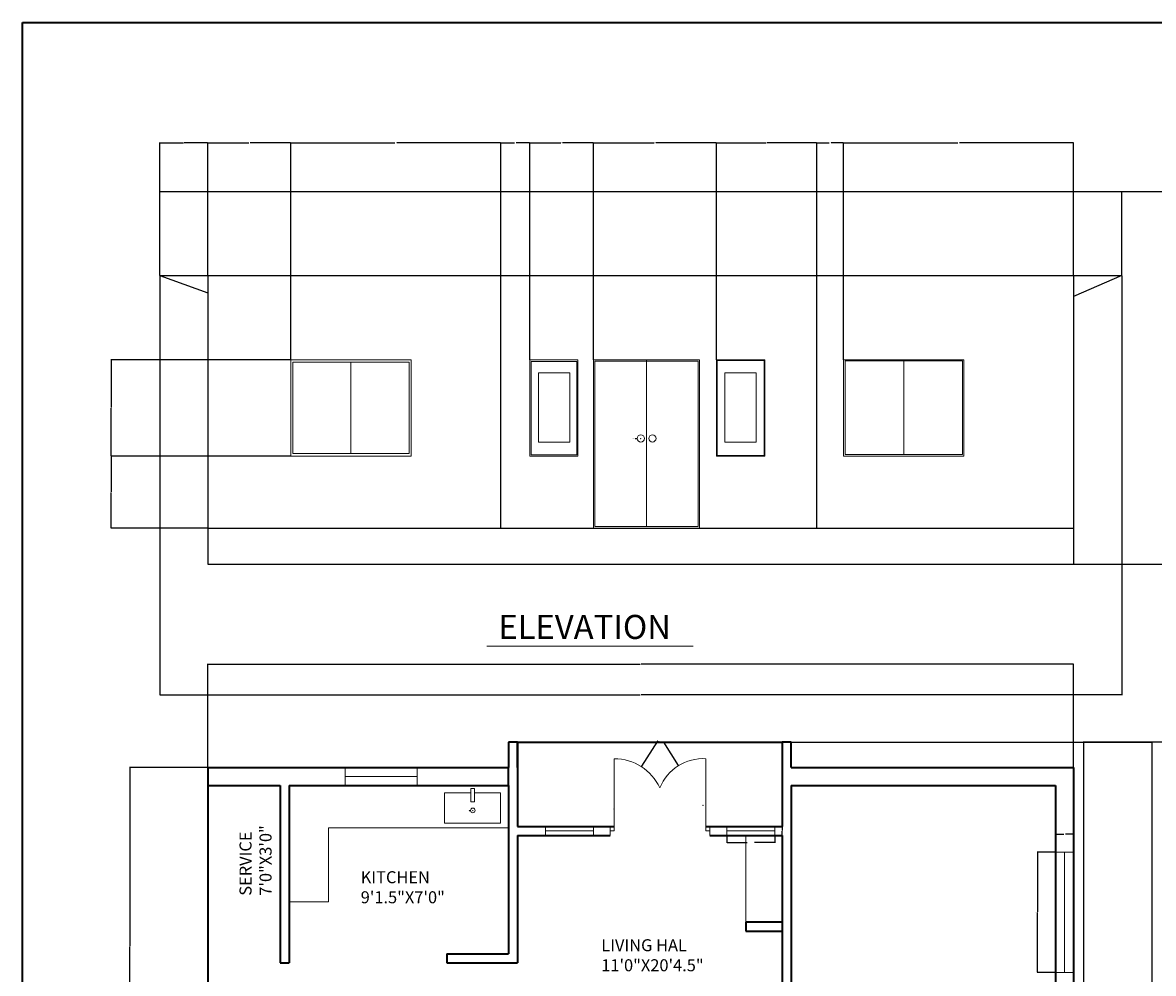
# Model space of a CAD drawing. Units: inches. Extents: x 2250 to 3547, y 1387 to 2604.
# Tile 3 of 11: x 2250 to 2814, y 2130 to 2604. Entities that reach past the tile are written whole.
import ezdxf

# ---------------------------------------------------------------- set-up
doc = ezdxf.new("R2010")
doc.units = ezdxf.units.IN
for name, color, linetype, lineweight in [('A-ANNO-DIMS', 2, 'Continuous', 18), ('A-ANNO-TEXT', 7, 'Continuous', 18), ('A-ANNO-TTLB', 7, 'Continuous', 35), ('A-AREA-IDEN', 7, 'Continuous', 18), ('A-DOOR', 3, 'Continuous', 18), ('A-ELEV', 7, 'Continuous', 25), ('A-FLOR-CASE', 9, 'Continuous', 18), ('A-FLOR-FIXT', 8, 'Continuous', 18), ('A-GLAZ', 4, 'Continuous', 18), ('A-WALL', 7, 'Continuous', 35)]:
    doc.layers.add(name, color=color, linetype=linetype, lineweight=lineweight)
doc.styles.get("Standard").update_dxf_attribs({"font": 'arial.ttf'})
doc.dimstyles.get("Standard").update_dxf_attribs({"dimtxt": 0.18, "dimasz": 0.18, "dimexe": 0.18, "dimexo": 0.0625, "dimgap": 0.09, "dimtad": 0, "dimtih": 1, "dimtoh": 1, "dimdec": 4, "dimzin": 0, "dimdsep": 46, "dimtxsty": 'Standard', "dimcen": 0.09, "dimadec": 0, "dimazin": 0, "dimtfac": 1, "dimtdec": 4, "dimtofl": 0, "dimtmove": 0, "dimatfit": 3, "dimfxl": 1, "dimtolj": 1, "dimtzin": 0, "dimarcsym": 0})

# ---------------------------------------------------------------- blocks, each defined once
blk = doc.blocks.new('WIN-24-SHALLOW')
for p, q in [((0, 4.5), (0, 0)), ((0, 0), (0, 2.25)), ((0, 2.25), (24, 2.25)), ((24, 2.25), (24, 4.5)), ((24, 4.5), (24, 0))]:
    blk.add_line(p, q)
blk = doc.blocks.new('WIN-36')
for p, q in [((0, 9), (0, 0)), ((36, 4.5), (36, 9)), ((36, 9), (36, 0)), ((0, 0), (0, 4.5)), ((0, 4.5), (36, 4.5))]:
    blk.add_line(p, q)
blk = doc.blocks.new('WIN-60-ALT-JAMB')
for p, q in [((9, 60), (0, 60)), ((0, 60), (4.5, 60)), ((4.5, 60), (4.5, 0)), ((4.5, 0), (0, 0)), ((0, 0), (9, 0))]:
    blk.add_line(p, q)
blk = doc.blocks.new('DOOR-ENTRY-DOUBLE-NORTH')
for p, q in [((2, 2.25), (2, 38.25)), ((47.76, 2.25), (47.76, 38.25)), ((0, 4.5), (0, 0)), ((0, 0), (0, 2.25)), ((0, 2.25), (2, 2.25)), ((49.76, 2.25), (47.76, 2.25)), ((49.76, 4.5), (49.76, 0)), ((49.76, 0), (49.76, 2.25))]:
    blk.add_line(p, q)
for centre, radius, start, end in [((2, 13.14), 25.11, 25.0388, 90), ((46.3, 15.04), 23.26, 86.4027, 157.9547)]:
    blk.add_arc(centre, radius, start, end)
blk = doc.blocks.new('KITCHEN-SINK-SINGLE')
blk.add_lwpolyline([(14.98, 17.19), (13.12, 17.19), (13.12, 10.67), (14.98, 10.67)], close=True)
blk.add_lwpolyline([(14.98, 15.02), (27.83, 15.02), (27.83, 0), (0, 0), (0, 15.02), (13.12, 15.02)])
blk.add_circle((14.09, 6.33), 1.15)
blk = doc.blocks.new('COUNTER-KITCHEN-N')
for p, q in [((19.63, 0), (19.63, 36.95)), ((19.63, 36.95), (109.5, 36.95)), ((0, 0), (19.63, 0))]:
    blk.add_line(p, q)
blk = doc.blocks.new('*D30')
at = {"layer": 'A-ANNO-DIMS', "color": 0, "lineweight": -2, "transparency": 16777216}
for p, q in [((2601.46, 2198.61), (2601.46, 2194.9)), ((2601.64, 2195.08), (2611.7, 2195.08)), ((2625.28, 2195.08), (2615.23, 2195.08)), ((2625.46, 2198.61), (2625.46, 2194.9))]:
    blk.add_line(p, q, dxfattribs=at)
at = {"layer": 'A-ANNO-DIMS', "color": 0, "transparency": 16777216}
for points in [[(2601.64, 2195.11), (2601.64, 2195.05), (2601.46, 2195.08)], [(2625.28, 2195.11), (2625.28, 2195.05), (2625.46, 2195.08)]]:
    blk.add_solid(points, dxfattribs=at)
at = {"layer": 'Defpoints', "color": 0, "transparency": 16777216}
for p in [(2601.46, 2198.68), (2625.46, 2198.68), (2625.46, 2195.08)]:
    blk.add_point(p, dxfattribs=at)
at = {"layer": 'A-ANNO-DIMS', "color": 0, "transparency": 16777216, "insert": (2613.46, 2195.08), "char_height": 0.18, "attachment_point": 5}
blk.add_mtext('\\A1;SHALLOW WINDOW 24 TYP.', dxfattribs=at)
blk = doc.blocks.new('*D31')
at = {"layer": 'A-ANNO-DIMS', "color": 0, "lineweight": -2, "transparency": 16777216}
for p, q in [((2625.53, 2203.18), (2629.24, 2203.18)), ((2629.06, 2203), (2629.06, 2201.11)), ((2629.06, 2198.86), (2629.06, 2200.74)), ((2625.53, 2198.68), (2629.24, 2198.68))]:
    blk.add_line(p, q, dxfattribs=at)
at = {"layer": 'A-ANNO-DIMS', "color": 0, "transparency": 16777216}
for points in [[(2629.03, 2203), (2629.09, 2203), (2629.06, 2203.18)], [(2629.03, 2198.86), (2629.09, 2198.86), (2629.06, 2198.68)]]:
    blk.add_solid(points, dxfattribs=at)
at = {"layer": 'Defpoints', "color": 0, "transparency": 16777216}
for p in [(2625.46, 2203.18), (2629.06, 2203.18), (2625.46, 2198.68)]:
    blk.add_point(p, dxfattribs=at)
at = {"layer": 'A-ANNO-DIMS', "color": 0, "transparency": 16777216, "insert": (2629.06, 2200.93), "char_height": 0.18, "attachment_point": 5}
blk.add_mtext('\\A1;5 TYP.', dxfattribs=at)
blk = doc.blocks.new('*D36')
at = {"layer": 'A-ANNO-DIMS', "color": 0, "lineweight": -2, "transparency": 16777216}
for p, q in [((2765.48, 2190.34), (2756.36, 2190.34)), ((2756.54, 2190.16), (2756.54, 2160.52)), ((2756.54, 2130.52), (2756.54, 2160.16)), ((2765.48, 2130.34), (2756.36, 2130.34))]:
    blk.add_line(p, q, dxfattribs=at)
at = {"layer": 'A-ANNO-DIMS', "color": 0, "transparency": 16777216}
for points in [[(2756.51, 2190.16), (2756.57, 2190.16), (2756.54, 2190.34)], [(2756.51, 2130.52), (2756.57, 2130.52), (2756.54, 2130.34)]]:
    blk.add_solid(points, dxfattribs=at)
at = {"layer": 'Defpoints', "color": 0, "transparency": 16777216}
for p in [(2756.54, 2190.34), (2765.54, 2190.34), (2765.54, 2130.34)]:
    blk.add_point(p, dxfattribs=at)
at = {"layer": 'A-ANNO-DIMS', "color": 0, "transparency": 16777216, "insert": (2756.54, 2160.34), "char_height": 0.18, "attachment_point": 5}
blk.add_mtext('\\A1;ALT. JAMB 60 TYP.', dxfattribs=at)
blk = doc.blocks.new('*D37')
at = {"layer": 'A-ANNO-DIMS', "color": 0, "lineweight": -2, "transparency": 16777216}
for p, q in [((2765.54, 2190.4), (2765.54, 2199.52)), ((2765.72, 2199.34), (2769.58, 2199.34)), ((2774.36, 2199.34), (2770.5, 2199.34)), ((2774.54, 2190.4), (2774.54, 2199.52))]:
    blk.add_line(p, q, dxfattribs=at)
at = {"layer": 'A-ANNO-DIMS', "color": 0, "transparency": 16777216}
for points in [[(2765.72, 2199.37), (2765.72, 2199.31), (2765.54, 2199.34)], [(2774.36, 2199.37), (2774.36, 2199.31), (2774.54, 2199.34)]]:
    blk.add_solid(points, dxfattribs=at)
at = {"layer": 'Defpoints', "color": 0, "transparency": 16777216}
for p in [(2774.54, 2199.34), (2765.54, 2190.34), (2774.54, 2190.34)]:
    blk.add_point(p, dxfattribs=at)
at = {"layer": 'A-ANNO-DIMS', "color": 0, "transparency": 16777216, "insert": (2770.04, 2199.34), "char_height": 0.18, "attachment_point": 5}
blk.add_mtext('\\A1;9 TYP.', dxfattribs=at)
blk = doc.blocks.new('*D76')
at = {"layer": 'A-ANNO-DIMS', "color": 0, "lineweight": -2, "transparency": 16777216}
for p, q in [((2342.54, 2232.63), (2342.54, 2284.31)), ((2342.72, 2284.13), (2558.25, 2284.13)), ((2774.36, 2284.13), (2558.83, 2284.13)), ((2774.54, 2232.63), (2774.54, 2284.31))]:
    blk.add_line(p, q, dxfattribs=at)
at = {"layer": 'A-ANNO-DIMS', "color": 0, "transparency": 16777216}
for points in [[(2342.72, 2284.16), (2342.72, 2284.1), (2342.54, 2284.13)], [(2774.36, 2284.16), (2774.36, 2284.1), (2774.54, 2284.13)]]:
    blk.add_solid(points, dxfattribs=at)
at = {"layer": 'Defpoints', "color": 0, "transparency": 16777216}
for p in [(2774.54, 2284.13), (2342.54, 2232.56), (2774.54, 2232.56)]:
    blk.add_point(p, dxfattribs=at)
at = {"layer": 'A-ANNO-DIMS', "color": 0, "transparency": 16777216, "insert": (2558.54, 2284.13), "char_height": 0.18, "attachment_point": 5}
blk.add_mtext('\\A1;432', dxfattribs=at)
blk = doc.blocks.new('*D77')
at = {"layer": 'A-ANNO-DIMS', "color": 0, "lineweight": -2, "transparency": 16777216}
for p, q in [((2633.6, 2245.18), (2813.67, 2245.18)), ((2813.49, 2245), (2813.49, 1894.73)), ((2813.49, 1544.1), (2813.49, 1894.37)), ((2774.6, 1543.92), (2813.67, 1543.92))]:
    blk.add_line(p, q, dxfattribs=at)
at = {"layer": 'A-ANNO-DIMS', "color": 0, "transparency": 16777216}
for points in [[(2813.46, 2245), (2813.52, 2245), (2813.49, 2245.18)], [(2813.46, 1544.1), (2813.52, 1544.1), (2813.49, 1543.92)]]:
    blk.add_solid(points, dxfattribs=at)
at = {"layer": 'Defpoints', "color": 0, "transparency": 16777216}
for p in [(2633.54, 2245.18), (2813.49, 2245.18), (2774.54, 1543.92)]:
    blk.add_point(p, dxfattribs=at)
at = {"layer": 'A-ANNO-DIMS', "color": 0, "transparency": 16777216, "insert": (2813.49, 1894.55), "char_height": 0.18, "attachment_point": 5}
blk.add_mtext('\\A1;701.3', dxfattribs=at)
blk = doc.blocks.new('*D83')
at = {"layer": 'A-ANNO-DIMS', "color": 0, "lineweight": -2, "transparency": 16777216}
for p, q in [((2342.48, 2232.56), (2303.41, 2232.56)), ((2303.59, 2232.38), (2303.59, 2143.51)), ((2303.59, 2054.27), (2303.59, 2143.15)), ((2342.48, 2054.09), (2303.41, 2054.09))]:
    blk.add_line(p, q, dxfattribs=at)
at = {"layer": 'A-ANNO-DIMS', "color": 0, "transparency": 16777216}
for points in [[(2303.56, 2232.38), (2303.62, 2232.38), (2303.59, 2232.56)], [(2303.56, 2054.27), (2303.62, 2054.27), (2303.59, 2054.09)]]:
    blk.add_solid(points, dxfattribs=at)
at = {"layer": 'Defpoints', "color": 0, "transparency": 16777216}
for p in [(2303.59, 2232.56), (2342.54, 2232.56), (2342.54, 2054.09)]:
    blk.add_point(p, dxfattribs=at)
at = {"layer": 'A-ANNO-DIMS', "color": 0, "transparency": 16777216, "insert": (2303.59, 2143.33), "char_height": 0.18, "attachment_point": 5}
blk.add_mtext('\\A1;178.47', dxfattribs=at)
blk = doc.blocks.new('*D85')
at = {"layer": 'A-ANNO-DIMS', "color": 0, "lineweight": -2, "transparency": 16777216}
for p, q in [((3001.57, 2245.18), (2779.34, 2245.18)), ((2779.52, 2245), (2779.52, 1894.73)), ((2779.52, 1544.1), (2779.52, 1894.37)), ((2851.57, 1543.92), (2779.34, 1543.92))]:
    blk.add_line(p, q, dxfattribs=at)
at = {"layer": 'A-ANNO-DIMS', "color": 0, "transparency": 16777216}
for points in [[(2779.49, 2245), (2779.55, 2245), (2779.52, 2245.18)], [(2779.49, 1544.1), (2779.55, 1544.1), (2779.52, 1543.92)]]:
    blk.add_solid(points, dxfattribs=at)
at = {"layer": 'Defpoints', "color": 0, "transparency": 16777216}
for p in [(2779.52, 2245.18), (3001.63, 2245.18), (2851.63, 1543.92)]:
    blk.add_point(p, dxfattribs=at)
at = {"layer": 'A-ANNO-DIMS', "color": 0, "transparency": 16777216, "insert": (2779.52, 1894.55), "char_height": 0.18, "attachment_point": 5}
blk.add_mtext('\\A1;701.3', dxfattribs=at)
blk = doc.blocks.new('*D95')
at = {"layer": 'A-ANNO-DIMS', "color": 0, "lineweight": -2, "transparency": 16777216}
for p, q in [((2318.54, 2477.89), (2318.54, 2268.64)), ((2798.54, 2477.89), (2798.54, 2268.64)), ((2318.72, 2268.82), (2558.25, 2268.82)), ((2798.36, 2268.82), (2558.83, 2268.82))]:
    blk.add_line(p, q, dxfattribs=at)
at = {"layer": 'A-ANNO-DIMS', "color": 0, "transparency": 16777216}
for points in [[(2318.72, 2268.85), (2318.72, 2268.79), (2318.54, 2268.82)], [(2798.36, 2268.85), (2798.36, 2268.79), (2798.54, 2268.82)]]:
    blk.add_solid(points, dxfattribs=at)
at = {"layer": 'Defpoints', "color": 0, "transparency": 16777216}
for p in [(2318.54, 2477.95), (2798.54, 2477.95), (2798.54, 2268.82)]:
    blk.add_point(p, dxfattribs=at)
at = {"layer": 'A-ANNO-DIMS', "color": 0, "transparency": 16777216, "insert": (2558.54, 2268.82), "char_height": 0.18, "attachment_point": 5}
blk.add_mtext('\\A1;480', dxfattribs=at)
blk = doc.blocks.new('*D96')
at = {"layer": 'A-ANNO-DIMS', "color": 0, "lineweight": -2, "transparency": 16777216}
for p, q in [((2798.6, 2519.95), (2822.97, 2519.95)), ((2822.79, 2519.77), (2822.79, 2427.13)), ((2822.79, 2334.13), (2822.79, 2426.77)), ((2774.6, 2333.95), (2822.97, 2333.95))]:
    blk.add_line(p, q, dxfattribs=at)
at = {"layer": 'A-ANNO-DIMS', "color": 0, "transparency": 16777216}
for points in [[(2822.76, 2519.77), (2822.82, 2519.77), (2822.79, 2519.95)], [(2822.76, 2334.13), (2822.82, 2334.13), (2822.79, 2333.95)]]:
    blk.add_solid(points, dxfattribs=at)
at = {"layer": 'Defpoints', "color": 0, "transparency": 16777216}
for p in [(2798.54, 2519.95), (2822.79, 2519.95), (2774.54, 2333.95)]:
    blk.add_point(p, dxfattribs=at)
at = {"layer": 'A-ANNO-DIMS', "color": 0, "transparency": 16777216, "insert": (2822.79, 2426.95), "char_height": 0.18, "attachment_point": 5}
blk.add_mtext('\\A1;186', dxfattribs=at)
blk = doc.blocks.new('*D97')
at = {"layer": 'A-ANNO-DIMS', "color": 0, "lineweight": -2, "transparency": 16777216}
for p, q in [((2383.88, 2387.95), (2294.11, 2387.95)), ((2294.29, 2387.77), (2294.29, 2370.13)), ((2294.29, 2352.13), (2294.29, 2369.77)), ((2342.48, 2351.95), (2294.11, 2351.95))]:
    blk.add_line(p, q, dxfattribs=at)
at = {"layer": 'A-ANNO-DIMS', "color": 0, "transparency": 16777216}
for points in [[(2294.26, 2387.77), (2294.32, 2387.77), (2294.29, 2387.95)], [(2294.26, 2352.13), (2294.32, 2352.13), (2294.29, 2351.95)]]:
    blk.add_solid(points, dxfattribs=at)
at = {"layer": 'Defpoints', "color": 0, "transparency": 16777216}
for p in [(2294.29, 2387.95), (2383.94, 2387.95), (2342.54, 2351.95)]:
    blk.add_point(p, dxfattribs=at)
at = {"layer": 'A-ANNO-DIMS', "color": 0, "transparency": 16777216, "insert": (2294.29, 2369.95), "char_height": 0.18, "attachment_point": 5}
blk.add_mtext('\\A1;36', dxfattribs=at)
blk = doc.blocks.new('*D98')
at = {"layer": 'A-ANNO-DIMS', "color": 0, "lineweight": -2, "transparency": 16777216}
for p, q in [((2383.88, 2435.95), (2294.11, 2435.95)), ((2294.29, 2435.77), (2294.29, 2412.13)), ((2294.29, 2388.13), (2294.29, 2411.77)), ((2383.88, 2387.95), (2294.11, 2387.95))]:
    blk.add_line(p, q, dxfattribs=at)
at = {"layer": 'A-ANNO-DIMS', "color": 0, "transparency": 16777216}
for points in [[(2294.26, 2435.77), (2294.32, 2435.77), (2294.29, 2435.95)], [(2294.26, 2388.13), (2294.32, 2388.13), (2294.29, 2387.95)]]:
    blk.add_solid(points, dxfattribs=at)
at = {"layer": 'Defpoints', "color": 0, "transparency": 16777216}
for p in [(2294.29, 2435.95), (2383.94, 2435.95), (2383.94, 2387.95)]:
    blk.add_point(p, dxfattribs=at)
at = {"layer": 'A-ANNO-DIMS', "color": 0, "transparency": 16777216, "insert": (2294.29, 2411.95), "char_height": 0.18, "attachment_point": 5}
blk.add_mtext('\\A1;48', dxfattribs=at)
blk = doc.blocks.new('*D99')
at = {"layer": 'A-ANNO-DIMS', "color": 0, "lineweight": -2, "transparency": 16777216}
for p, q in [((2318.54, 2520.01), (2318.54, 2544.38)), ((2318.72, 2544.2), (2330.32, 2544.2)), ((2342.36, 2544.2), (2330.76, 2544.2)), ((2342.54, 2478.01), (2342.54, 2544.38))]:
    blk.add_line(p, q, dxfattribs=at)
at = {"layer": 'A-ANNO-DIMS', "color": 0, "transparency": 16777216}
for points in [[(2318.72, 2544.23), (2318.72, 2544.17), (2318.54, 2544.2)], [(2342.36, 2544.23), (2342.36, 2544.17), (2342.54, 2544.2)]]:
    blk.add_solid(points, dxfattribs=at)
at = {"layer": 'Defpoints', "color": 0, "transparency": 16777216}
for p in [(2342.54, 2544.2), (2318.54, 2519.95), (2342.54, 2477.95)]:
    blk.add_point(p, dxfattribs=at)
at = {"layer": 'A-ANNO-DIMS', "color": 0, "transparency": 16777216, "insert": (2330.54, 2544.2), "char_height": 0.18, "attachment_point": 5}
blk.add_mtext('\\A1;24', dxfattribs=at)
blk = doc.blocks.new('*D100')
at = {"layer": 'A-ANNO-DIMS', "color": 0, "lineweight": -2, "transparency": 16777216}
for p, q in [((2342.54, 2478.01), (2342.54, 2544.38)), ((2342.72, 2544.2), (2362.91, 2544.2)), ((2383.76, 2544.2), (2363.57, 2544.2)), ((2383.94, 2436.01), (2383.94, 2544.38))]:
    blk.add_line(p, q, dxfattribs=at)
at = {"layer": 'A-ANNO-DIMS', "color": 0, "transparency": 16777216}
for points in [[(2342.72, 2544.23), (2342.72, 2544.17), (2342.54, 2544.2)], [(2383.76, 2544.23), (2383.76, 2544.17), (2383.94, 2544.2)]]:
    blk.add_solid(points, dxfattribs=at)
at = {"layer": 'Defpoints', "color": 0, "transparency": 16777216}
for p in [(2383.94, 2544.2), (2342.54, 2477.95), (2383.94, 2435.95)]:
    blk.add_point(p, dxfattribs=at)
at = {"layer": 'A-ANNO-DIMS', "color": 0, "transparency": 16777216, "insert": (2363.24, 2544.2), "char_height": 0.18, "attachment_point": 5}
blk.add_mtext('\\A1;41.4', dxfattribs=at)
blk = doc.blocks.new('*D101')
at = {"layer": 'A-ANNO-DIMS', "color": 0, "lineweight": -2, "transparency": 16777216}
for p, q in [((2383.94, 2436.01), (2383.94, 2544.38)), ((2384.12, 2544.2), (2435.87, 2544.2)), ((2488.54, 2544.2), (2436.78, 2544.2)), ((2488.72, 2478.01), (2488.72, 2544.38))]:
    blk.add_line(p, q, dxfattribs=at)
at = {"layer": 'A-ANNO-DIMS', "color": 0, "transparency": 16777216}
for points in [[(2384.12, 2544.23), (2384.12, 2544.17), (2383.94, 2544.2)], [(2488.54, 2544.23), (2488.54, 2544.17), (2488.72, 2544.2)]]:
    blk.add_solid(points, dxfattribs=at)
at = {"layer": 'Defpoints', "color": 0, "transparency": 16777216}
for p in [(2488.72, 2544.2), (2488.72, 2477.95), (2383.94, 2435.95)]:
    blk.add_point(p, dxfattribs=at)
at = {"layer": 'A-ANNO-DIMS', "color": 0, "transparency": 16777216, "insert": (2436.33, 2544.2), "char_height": 0.18, "attachment_point": 5}
blk.add_mtext('\\A1;104.78', dxfattribs=at)
blk = doc.blocks.new('*D102')
at = {"layer": 'A-ANNO-DIMS', "color": 0, "lineweight": -2, "transparency": 16777216}
for p, q in [((2488.72, 2478.01), (2488.72, 2544.38)), ((2488.9, 2544.2), (2495.49, 2544.2)), ((2502.99, 2544.2), (2496.4, 2544.2)), ((2503.17, 2436.01), (2503.17, 2544.38))]:
    blk.add_line(p, q, dxfattribs=at)
at = {"layer": 'A-ANNO-DIMS', "color": 0, "transparency": 16777216}
for points in [[(2488.9, 2544.23), (2488.9, 2544.17), (2488.72, 2544.2)], [(2502.99, 2544.23), (2502.99, 2544.17), (2503.17, 2544.2)]]:
    blk.add_solid(points, dxfattribs=at)
at = {"layer": 'Defpoints', "color": 0, "transparency": 16777216}
for p in [(2503.17, 2544.2), (2488.72, 2477.95), (2503.17, 2435.95)]:
    blk.add_point(p, dxfattribs=at)
at = {"layer": 'A-ANNO-DIMS', "color": 0, "transparency": 16777216, "insert": (2495.94, 2544.2), "char_height": 0.18, "attachment_point": 5}
blk.add_mtext('\\A1;14.453', dxfattribs=at)
blk = doc.blocks.new('*D103')
at = {"layer": 'A-ANNO-DIMS', "color": 0, "lineweight": -2, "transparency": 16777216}
for p, q in [((2503.17, 2436.01), (2503.17, 2544.38)), ((2503.35, 2544.2), (2518.64, 2544.2)), ((2534.72, 2544.2), (2519.43, 2544.2)), ((2534.9, 2436.01), (2534.9, 2544.38))]:
    blk.add_line(p, q, dxfattribs=at)
at = {"layer": 'A-ANNO-DIMS', "color": 0, "transparency": 16777216}
for points in [[(2503.35, 2544.23), (2503.35, 2544.17), (2503.17, 2544.2)], [(2534.72, 2544.23), (2534.72, 2544.17), (2534.9, 2544.2)]]:
    blk.add_solid(points, dxfattribs=at)
at = {"layer": 'Defpoints', "color": 0, "transparency": 16777216}
for p in [(2534.9, 2544.2), (2503.17, 2435.95), (2534.9, 2435.95)]:
    blk.add_point(p, dxfattribs=at)
at = {"layer": 'A-ANNO-DIMS', "color": 0, "transparency": 16777216, "insert": (2519.04, 2544.2), "char_height": 0.18, "attachment_point": 5}
blk.add_mtext('\\A1;31.73', dxfattribs=at)
blk = doc.blocks.new('*D104')
at = {"layer": 'A-ANNO-DIMS', "color": 0, "lineweight": -2, "transparency": 16777216}
for p, q in [((2534.9, 2436.01), (2534.9, 2544.38)), ((2535.08, 2544.2), (2565.24, 2544.2)), ((2596.19, 2544.2), (2566.03, 2544.2)), ((2596.37, 2436.01), (2596.37, 2544.38))]:
    blk.add_line(p, q, dxfattribs=at)
at = {"layer": 'A-ANNO-DIMS', "color": 0, "transparency": 16777216}
for points in [[(2535.08, 2544.23), (2535.08, 2544.17), (2534.9, 2544.2)], [(2596.19, 2544.23), (2596.19, 2544.17), (2596.37, 2544.2)]]:
    blk.add_solid(points, dxfattribs=at)
at = {"layer": 'Defpoints', "color": 0, "transparency": 16777216}
for p in [(2596.37, 2544.2), (2534.9, 2435.95), (2596.37, 2435.95)]:
    blk.add_point(p, dxfattribs=at)
at = {"layer": 'A-ANNO-DIMS', "color": 0, "transparency": 16777216, "insert": (2565.64, 2544.2), "char_height": 0.18, "attachment_point": 5}
blk.add_mtext('\\A1;61.47', dxfattribs=at)
blk = doc.blocks.new('*D105')
at = {"layer": 'A-ANNO-DIMS', "color": 0, "lineweight": -2, "transparency": 16777216}
for p, q in [((2596.37, 2436.01), (2596.37, 2544.38)), ((2596.55, 2544.2), (2621.16, 2544.2)), ((2646.2, 2544.2), (2621.59, 2544.2)), ((2646.38, 2478.01), (2646.38, 2544.38))]:
    blk.add_line(p, q, dxfattribs=at)
at = {"layer": 'A-ANNO-DIMS', "color": 0, "transparency": 16777216}
for points in [[(2596.55, 2544.23), (2596.55, 2544.17), (2596.37, 2544.2)], [(2646.2, 2544.23), (2646.2, 2544.17), (2646.38, 2544.2)]]:
    blk.add_solid(points, dxfattribs=at)
at = {"layer": 'Defpoints', "color": 0, "transparency": 16777216}
for p in [(2646.38, 2544.2), (2646.38, 2477.95), (2596.37, 2435.95)]:
    blk.add_point(p, dxfattribs=at)
at = {"layer": 'A-ANNO-DIMS', "color": 0, "transparency": 16777216, "insert": (2621.37, 2544.2), "char_height": 0.18, "attachment_point": 5}
blk.add_mtext('\\A1;50', dxfattribs=at)
blk = doc.blocks.new('*D106')
at = {"layer": 'A-ANNO-DIMS', "color": 0, "lineweight": -2, "transparency": 16777216}
for p, q in [((2646.38, 2478.01), (2646.38, 2544.38)), ((2646.56, 2544.2), (2652.61, 2544.2)), ((2659.56, 2544.2), (2653.52, 2544.2)), ((2659.74, 2436.01), (2659.74, 2544.38))]:
    blk.add_line(p, q, dxfattribs=at)
at = {"layer": 'A-ANNO-DIMS', "color": 0, "transparency": 16777216}
for points in [[(2646.56, 2544.23), (2646.56, 2544.17), (2646.38, 2544.2)], [(2659.56, 2544.23), (2659.56, 2544.17), (2659.74, 2544.2)]]:
    blk.add_solid(points, dxfattribs=at)
at = {"layer": 'Defpoints', "color": 0, "transparency": 16777216}
for p in [(2659.74, 2544.2), (2646.38, 2477.95), (2659.74, 2435.95)]:
    blk.add_point(p, dxfattribs=at)
at = {"layer": 'A-ANNO-DIMS', "color": 0, "transparency": 16777216, "insert": (2653.06, 2544.2), "char_height": 0.18, "attachment_point": 5}
blk.add_mtext('\\A1;13.367', dxfattribs=at)
blk = doc.blocks.new('*D107')
at = {"layer": 'A-ANNO-DIMS', "color": 0, "lineweight": -2, "transparency": 16777216}
for p, q in [((2659.74, 2436.01), (2659.74, 2544.38)), ((2659.92, 2544.2), (2716.76, 2544.2)), ((2774.36, 2544.2), (2717.53, 2544.2)), ((2774.54, 2478.01), (2774.54, 2544.38))]:
    blk.add_line(p, q, dxfattribs=at)
at = {"layer": 'A-ANNO-DIMS', "color": 0, "transparency": 16777216}
for points in [[(2659.92, 2544.23), (2659.92, 2544.17), (2659.74, 2544.2)], [(2774.36, 2544.23), (2774.36, 2544.17), (2774.54, 2544.2)]]:
    blk.add_solid(points, dxfattribs=at)
at = {"layer": 'Defpoints', "color": 0, "transparency": 16777216}
for p in [(2774.54, 2544.2), (2774.54, 2477.95), (2659.74, 2435.95)]:
    blk.add_point(p, dxfattribs=at)
at = {"layer": 'A-ANNO-DIMS', "color": 0, "transparency": 16777216, "insert": (2717.14, 2544.2), "char_height": 0.18, "attachment_point": 5}
blk.add_mtext('\\A1;114.8', dxfattribs=at)
blk = doc.blocks.new('*D125')
at = {"layer": 'A-ANNO-DIMS', "color": 0, "lineweight": -2, "transparency": 16777216}
for p, q in [((2566.9, 2245.71), (2558.91, 2233.15)), ((2567.08, 2245.71), (2566.9, 2245.71)), ((2545.24, 2211.82), (2545.42, 2211.82)), ((2545.33, 2211.73), (2545.33, 2211.91))]:
    blk.add_line(p, q, dxfattribs=at)
at = {"layer": 'A-ANNO-DIMS', "color": 0, "transparency": 16777216}
blk.add_solid([(2558.88, 2233.17), (2558.93, 2233.13), (2558.81, 2233)], dxfattribs=at)
at = {"layer": 'Defpoints', "color": 0, "transparency": 16777216}
for p in [(2558.81, 2233), (2545.33, 2211.82)]:
    blk.add_point(p, dxfattribs=at)
at = {"layer": 'A-ANNO-DIMS', "color": 0, "transparency": 16777216, "insert": (2567.54, 2245.71), "char_height": 0.18, "attachment_point": 5}
blk.add_mtext('\\A1;R25.11', dxfattribs=at)
blk = doc.blocks.new('*D127')
at = {"layer": 'A-ANNO-DIMS', "color": 0, "lineweight": -2, "transparency": 16777216}
for p, q in [((2569.63, 2245.21), (2569.81, 2245.21)), ((2569.81, 2245.21), (2577.15, 2233.55)), ((2589.54, 2213.72), (2589.72, 2213.72)), ((2589.63, 2213.63), (2589.63, 2213.81))]:
    blk.add_line(p, q, dxfattribs=at)
at = {"layer": 'A-ANNO-DIMS', "color": 0, "transparency": 16777216}
blk.add_solid([(2577.17, 2233.57), (2577.12, 2233.54), (2577.25, 2233.4)], dxfattribs=at)
at = {"layer": 'Defpoints', "color": 0, "transparency": 16777216}
for p in [(2577.25, 2233.4), (2589.63, 2213.72)]:
    blk.add_point(p, dxfattribs=at)
at = {"layer": 'A-ANNO-DIMS', "color": 0, "transparency": 16777216, "insert": (2569.08, 2245.21), "char_height": 0.18, "attachment_point": 5}
blk.add_mtext('\\A1;R23.256', dxfattribs=at)
blk = doc.blocks.new('*D130')
at = {"layer": 'A-ANNO-DIMS', "color": 0, "lineweight": -2, "transparency": 16777216}
for p, q in [((2472.93, 2211.15), (2473.44, 2211.15)), ((2474.68, 2211.16), (2474.86, 2211.16)), ((2474.77, 2211.07), (2474.77, 2211.25))]:
    blk.add_line(p, q, dxfattribs=at)
at = {"layer": 'A-ANNO-DIMS', "color": 0, "transparency": 16777216}
blk.add_solid([(2473.44, 2211.18), (2473.44, 2211.12), (2473.62, 2211.15)], dxfattribs=at)
at = {"layer": 'Defpoints', "color": 0, "transparency": 16777216}
for p in [(2473.62, 2211.15), (2475.92, 2211.17)]:
    blk.add_point(p, dxfattribs=at)
at = {"layer": 'A-ANNO-DIMS', "color": 0, "transparency": 16777216, "insert": (2472.24, 2211.15), "char_height": 0.18, "attachment_point": 5}
blk.add_mtext('\\A1;2X ∅2.303', dxfattribs=at)
blk = doc.blocks.new('*D131')
at = {"layer": 'A-ANNO-DIMS', "color": 0, "lineweight": -2, "transparency": 16777216}
for p, q in [((2555.69, 2396.75), (2556.59, 2396.75)), ((2558.48, 2396.75), (2558.66, 2396.75)), ((2558.57, 2396.66), (2558.57, 2396.84))]:
    blk.add_line(p, q, dxfattribs=at)
at = {"layer": 'A-ANNO-DIMS', "color": 0, "transparency": 16777216}
blk.add_solid([(2556.59, 2396.78), (2556.59, 2396.72), (2556.77, 2396.75)], dxfattribs=at)
at = {"layer": 'Defpoints', "color": 0, "transparency": 16777216}
for p in [(2556.77, 2396.75), (2560.37, 2396.75)]:
    blk.add_point(p, dxfattribs=at)
at = {"layer": 'A-ANNO-DIMS', "color": 0, "transparency": 16777216, "insert": (2555, 2396.75), "char_height": 0.18, "attachment_point": 5}
blk.add_mtext('\\A1;2X ∅3.603', dxfattribs=at)

msp = doc.modelspace()

# ---------------------------------------------------------------- linework, layer by layer
at = {"layer": 'A-ANNO-TEXT'}
msp.add_line((2481.7495, 2293.0682), (2584.7527, 2293.0682), dxfattribs=at)
at = {"layer": 'A-ANNO-TTLB'}
msp.add_lwpolyline([(2250.1093, 2604.1988), (3546.995, 2604.1988), (3546.995, 1386.7251), (2250.1093, 1386.7251)], close=True, dxfattribs=at)
at = {"layer": 'A-DOOR'}
for p, q in [((2534.9015, 2435.9493), (2534.9015, 2351.9493)), ((2534.9015, 2435.9493), (2587.9248, 2435.9493)), ((2561.4131, 2435.9493), (2561.3878, 2352.7171)), ((2587.9248, 2435.9493), (2587.9248, 2351.9493))]:
    msp.add_line(p, q, dxfattribs=at)
msp.add_lwpolyline([(2535.6239, 2435.237), (2587.1517, 2435.237), (2587.1517, 2352.7171), (2535.6239, 2352.7171)], close=True, dxfattribs=at)
for centre in [(2558.5689, 2396.7486), (2564.3634, 2396.7486)]:
    msp.add_circle(centre, 1.8014, dxfattribs=at)
at = {"layer": 'A-ELEV'}
for p, q in [((2318.5378, 2519.9493), (2798.5378, 2519.9493)), ((2318.5378, 2477.9493), (2318.5378, 2519.9493)), ((2798.5378, 2477.9493), (2798.5378, 2519.9493)), ((2318.5378, 2477.9493), (2798.5378, 2477.9493)), ((2318.5378, 2477.9493), (2342.5378, 2469.3276)), ((2342.5378, 2477.9493), (2342.5378, 2333.9493)), ((2488.7165, 2351.9493), (2488.7165, 2477.9493)), ((2646.3771, 2351.9493), (2646.3771, 2477.9493)), ((2774.5378, 2477.9493), (2774.5378, 2333.9493)), ((2798.5378, 2477.9493), (2774.5378, 2467.4902)), ((2342.5378, 2351.9493), (2774.5378, 2351.9493)), ((2342.5378, 2333.9493), (2774.5378, 2333.9493))]:
    msp.add_line(p, q, dxfattribs=at)
at = {"layer": 'A-FLOR-CASE'}
msp.add_line((2611.0328, 2155.4117), (2611.0328, 2198.6762), dxfattribs=at)
at = {"layer": 'A-GLAZ'}
for p, q in [((2383.9389, 2435.9493), (2383.9389, 2387.9493)), ((2383.9389, 2435.9493), (2443.9389, 2435.9493)), ((2413.8889, 2434.8418), (2413.8889, 2389.288)), ((2443.9389, 2435.9493), (2443.9389, 2387.9493)), ((2503.1695, 2435.9493), (2503.1695, 2387.9493)), ((2503.1695, 2435.9493), (2527.1695, 2435.9493)), ((2527.1695, 2435.9493), (2527.1695, 2387.9493)), ((2596.3725, 2435.9493), (2596.3725, 2387.9493)), ((2596.3725, 2435.9493), (2620.3725, 2435.9493)), ((2620.3725, 2435.9493), (2620.3725, 2387.9493)), ((2659.744, 2435.9493), (2659.744, 2387.9493)), ((2659.744, 2435.9493), (2719.744, 2435.9493)), ((2689.787, 2435.3824), (2689.787, 2388.7928)), ((2719.744, 2435.9493), (2719.744, 2387.9493)), ((2383.9389, 2387.9493), (2443.9389, 2387.9493)), ((2503.1695, 2387.9493), (2527.1695, 2387.9493)), ((2596.3725, 2387.9493), (2620.3725, 2387.9493)), ((2659.744, 2387.9493), (2719.744, 2387.9493))]:
    msp.add_line(p, q, dxfattribs=at)
for points in [[(2384.8703, 2434.8418), (2442.9075, 2434.8418), (2442.9075, 2389.288), (2384.8703, 2389.288)], [(2503.8783, 2435.1391), (2526.6814, 2435.1391), (2526.6814, 2388.4979), (2503.8783, 2388.4979)], [(2596.7444, 2435.6488), (2620.152, 2435.6488), (2620.152, 2388.1627), (2596.7444, 2388.1627)], [(2660.4863, 2435.3824), (2719.0877, 2435.3824), (2719.0877, 2388.7928), (2660.4863, 2388.7928)], [(2507.5123, 2429.5171), (2523.1453, 2429.5171), (2523.1453, 2394.9004), (2507.5123, 2394.9004)], [(2600.5297, 2429.5171), (2616.1627, 2429.5171), (2616.1627, 2394.9004), (2600.5297, 2394.9004)]]:
    msp.add_lwpolyline(points, close=True, dxfattribs=at)
at = {"layer": 'A-WALL'}
for p, q in [((2497.0378, 2245.1762), (2492.5378, 2245.1762)), ((2492.5378, 2245.1762), (2492.5378, 2232.5639)), ((2497.0378, 2245.1762), (2497.0378, 2203.1762)), ((2497.0378, 2232.5639), (2497.0378, 2245.1762)), ((2497.0378, 2245.1762), (2629.0378, 2245.1762)), ((2629.0378, 2245.1762), (2629.0378, 2203.1762)), ((2633.5378, 2245.1762), (2629.0378, 2245.1762)), ((2629.0378, 2245.1762), (2629.0378, 2232.5639)), ((2633.5378, 2232.5639), (2633.5378, 2245.1762)), ((2342.5378, 2232.5639), (2342.5378, 1899.5639)), ((2342.5378, 2232.5639), (2342.5378, 1899.5639)), ((2342.5378, 2232.5639), (2492.5378, 2232.5639)), ((2492.5378, 2223.5639), (2492.5378, 2232.5639)), ((2633.5378, 2232.5639), (2774.5378, 2232.5639)), ((2774.5378, 2232.5639), (2774.5378, 1543.9245)), ((2342.5378, 2223.5639), (2378.5378, 2223.5639)), ((2378.5378, 2223.5639), (2378.5378, 2135.0639)), ((2383.0378, 2223.5639), (2383.0378, 2135.0639)), ((2383.0378, 2223.5639), (2492.5378, 2223.5639)), ((2492.5378, 2223.5639), (2492.5378, 2139.5639)), ((2633.5378, 2223.5639), (2633.5378, 2094.5639)), ((2633.5378, 2223.5639), (2765.5378, 2223.5639)), ((2765.5378, 2223.5639), (2765.5378, 2094.5639)), ((2497.0378, 2203.1762), (2545.3262, 2203.1762)), ((2591.0889, 2203.1762), (2629.0378, 2203.1762)), ((2497.0378, 2198.6762), (2543.3262, 2198.6762)), ((2497.0378, 2198.6762), (2497.0378, 2135.0639)), ((2593.0889, 2198.6762), (2629.0378, 2198.6762)), ((2629.0378, 2198.6762), (2629.0378, 2090.0639)), ((2629.0378, 2155.4117), (2611.0328, 2155.4117)), ((2611.0328, 2155.4117), (2611.0328, 2150.9117)), ((2611.0328, 2150.9117), (2629.0378, 2150.9117)), ((2461.8375, 2139.5639), (2492.5378, 2139.5639)), ((2461.8375, 2139.5639), (2461.8375, 2135.0639)), ((2378.5378, 2135.0639), (2383.0378, 2135.0639)), ((2461.8375, 2135.0639), (2497.0378, 2135.0639))]:
    msp.add_line(p, q, dxfattribs=at)

# ---------------------------------------------------------------- block references
at = {"layer": 'A-DOOR'}
msp.add_blockref('DOOR-ENTRY-DOUBLE-NORTH', (2543.3262, 2198.6762), dxfattribs=at)
at = {"layer": 'A-FLOR-CASE'}
msp.add_blockref('COUNTER-KITCHEN-N', (2383.0378, 2165.4936), dxfattribs=at)
at = {"layer": 'A-FLOR-FIXT'}
msp.add_blockref('KITCHEN-SINK-SINGLE', (2460.6775, 2204.8244), dxfattribs=at)
at = {"layer": 'A-GLAZ'}
for name, p in [('WIN-36', (2411.0532, 2223.5639)), ('WIN-24-SHALLOW', (2601.4635, 2198.6762)), ('WIN-60-ALT-JAMB', (2765.5378, 2130.3411))]:
    msp.add_blockref(name, p, dxfattribs=at)
at = {"layer": 'A-GLAZ', "rotation": 180}
msp.add_blockref('WIN-24-SHALLOW', (2535.0378, 2203.1762), dxfattribs=at)

# ---------------------------------------------------------------- texts
at = {"layer": 'A-ANNO-TEXT', "insert": (2487.4869, 2308.6951), "char_height": 12, "attachment_point": 1}
msp.add_mtext_dynamic_manual_height_columns('ELEVATION', width=256.573617, gutter_width=12.5, heights=[0], dxfattribs=at)
at = {"layer": 'A-AREA-IDEN', "insert": (2358.3355, 2168.5837), "char_height": 6, "attachment_point": 1, "rotation": 90}
msp.add_mtext_dynamic_manual_height_columns('SERVICE \\P7\'0"X3\'0"', width=317.1373, gutter_width=12.5, heights=[0], dxfattribs=at)
at = {"layer": 'A-AREA-IDEN', "char_height": 6, "attachment_point": 1}
for s, width, insert in [('KITCHEN\\P9\'1.5"X7\'0"', 90.179104, (2418.8168, 2180.8149)), ('LIVING HAL\\P11\'0"X20\'4.5"', 48.207468, (2538.8416, 2146.887))]:
    msp.add_mtext_dynamic_manual_height_columns(s, width=width, gutter_width=12.5, heights=[0], dxfattribs=dict(at, insert=insert))

# ---------------------------------------------------------------- dimensions: what is measured, and where the dimension line sits
at = {"layer": 'A-ANNO-DIMS'}
for base, p1, p2, override, picture, middle in [((2342.5378, 2544.1993), (2318.5378, 2519.9493), (2342.5378, 2477.9493), {"dimdec": 0, "dimlfac": 1, "dimrnd": 0, "dimzin": 0, "dimdsep": 46, "dimlunit": 2}, '*D99', (2330.5378, 2544.1993)), ((2383.9389, 2544.1993), (2342.5378, 2477.9493), (2383.9389, 2435.9493), {"dimdec": 1, "dimlfac": 1, "dimrnd": 0, "dimzin": 0, "dimdsep": 46, "dimlunit": 2}, '*D100', (2363.2384, 2544.1993)), ((2488.7165, 2544.1993), (2383.9389, 2435.9493), (2488.7165, 2477.9493), {"dimdec": 2, "dimlfac": 1, "dimrnd": 0, "dimzin": 0, "dimdsep": 46, "dimlunit": 2}, '*D101', (2436.3277, 2544.1993)), ((2503.1695, 2544.1993), (2488.7165, 2477.9493), (2503.1695, 2435.9493), {"dimdec": 3, "dimlfac": 1, "dimrnd": 0, "dimzin": 0, "dimdsep": 46, "dimlunit": 2}, '*D102', (2495.943, 2544.1993)), ((2534.9015, 2544.1993), (2503.1695, 2435.9493), (2534.9015, 2435.9493), {"dimdec": 2, "dimlfac": 1, "dimrnd": 0, "dimzin": 0, "dimdsep": 46, "dimlunit": 2}, '*D103', (2519.0355, 2544.1993)), ((2596.3725, 2544.1993), (2534.9015, 2435.9493), (2596.3725, 2435.9493), {"dimdec": 2, "dimlfac": 1, "dimrnd": 0, "dimzin": 0, "dimdsep": 46, "dimlunit": 2}, '*D104', (2565.637, 2544.1993)), ((2646.3771, 2544.1993), (2596.3725, 2435.9493), (2646.3771, 2477.9493), {"dimdec": 0, "dimlfac": 1, "dimrnd": 0, "dimzin": 0, "dimdsep": 46, "dimlunit": 2}, '*D105', (2621.3748, 2544.1993)), ((2659.744, 2544.1993), (2646.3771, 2477.9493), (2659.744, 2435.9493), {"dimdec": 3, "dimlfac": 1, "dimrnd": 0, "dimzin": 0, "dimdsep": 46, "dimlunit": 2}, '*D106', (2653.0605, 2544.1993)), ((2774.5378, 2544.1993), (2659.744, 2435.9493), (2774.5378, 2477.9493), {"dimdec": 1, "dimlfac": 1, "dimrnd": 0, "dimzin": 0, "dimdsep": 46, "dimlunit": 2}, '*D107', (2717.1409, 2544.1993)), ((2798.5378, 2268.8182), (2318.5378, 2477.9493), (2798.5378, 2477.9493), {"dimdec": 0, "dimlfac": 1, "dimrnd": 0, "dimzin": 0, "dimdsep": 46, "dimlunit": 2}, '*D95', (2558.5378, 2268.8182)), ((2774.5378, 2284.1262), (2342.5378, 2232.5639), (2774.5378, 2232.5639), {"dimdec": 0, "dimlfac": 1, "dimrnd": 0, "dimzin": 0, "dimdsep": 46, "dimlunit": 2}, '*D76', (2558.5378, 2284.1262))]:
    dim = msp.add_linear_dim(base=base, p1=p1, p2=p2, dimstyle='Standard', override=override, dxfattribs=at)
    dim.commit()
    dim.dimension.update_dxf_attribs({"geometry": picture, "text_midpoint": middle})
for base, p1, p2, override, picture, middle in [((2822.7878, 2519.9493), (2774.5378, 2333.9493), (2798.5378, 2519.9493), {"dimdec": 0, "dimlfac": 1, "dimrnd": 0, "dimzin": 0, "dimdsep": 46, "dimlunit": 2}, '*D96', (2822.7878, 2426.9493)), ((2294.2878, 2435.9493), (2383.9389, 2387.9493), (2383.9389, 2435.9493), {"dimdec": 0, "dimlfac": 1, "dimrnd": 0, "dimzin": 0, "dimdsep": 46, "dimlunit": 2}, '*D98', (2294.2878, 2411.9493)), ((2294.2878, 2387.9493), (2342.5378, 2351.9493), (2383.9389, 2387.9493), {"dimdec": 0, "dimlfac": 1, "dimrnd": 0, "dimzin": 0, "dimdsep": 46, "dimlunit": 2}, '*D97', (2294.2878, 2369.9493)), ((2813.4878, 2245.1762), (2774.5378, 1543.9245), (2633.5378, 2245.1762), {"dimdec": 1, "dimlfac": 1, "dimrnd": 0, "dimzin": 0, "dimdsep": 46, "dimlunit": 2}, '*D77', (2813.4878, 1894.5504)), ((2779.5165, 2245.1762), (2851.6288, 1543.9245), (3001.6288, 2245.1762), {"dimdec": 1, "dimlfac": 1, "dimrnd": 0, "dimzin": 0, "dimdsep": 46, "dimlunit": 2}, '*D85', (2779.5165, 1894.5504)), ((2303.5878, 2232.5639), (2342.5378, 2054.091), (2342.5378, 2232.5639), {"dimdec": 2, "dimlfac": 1, "dimrnd": 0, "dimzin": 0, "dimdsep": 46, "dimlunit": 2}, '*D83', (2303.5878, 2143.3274))]:
    dim = msp.add_linear_dim(base=base, p1=p1, p2=p2, angle=90, dimstyle='Standard', override=override, dxfattribs=at)
    dim.commit()
    dim.dimension.update_dxf_attribs({"geometry": picture, "text_midpoint": middle})
for p1, p2, picture, middle in [((2560.3703, 2396.7473), (2556.7675, 2396.75), '*D131', (2555.6866, 2396.7508)), ((2475.9198, 2211.1663), (2473.6166, 2211.1501), '*D130', (2472.9257, 2211.1453))]:
    dim = msp.add_diameter_dim_2p(p1=p1, p2=p2, text='2X <>', dimstyle='Standard', override={"dimdec": 3, "dimlfac": 1, "dimrnd": 0, "dimzin": 0, "dimdsep": 46, "dimlunit": 2}, dxfattribs=at)
    dim.commit()
    dim.dimension.update_dxf_attribs({"geometry": picture, "text_midpoint": middle, "dimtype": 163})
for center, mpoint, override, picture, middle in [((2545.3262, 2211.8186), (2558.8089, 2232.9989), {"dimdec": 2, "dimlfac": 1, "dimrnd": 0, "dimzin": 0, "dimdsep": 46, "dimlunit": 2}, '*D125', (2567.541, 2245.7071)), ((2589.6298, 2213.7161), (2577.245, 2233.4), {"dimdec": 3, "dimlfac": 1, "dimrnd": 0, "dimzin": 0, "dimdsep": 46, "dimlunit": 2}, '*D127', (2569.0845, 2245.2103))]:
    dim = msp.add_radius_dim(center=center, mpoint=mpoint, dimstyle='Standard', override=override, dxfattribs=at)
    dim.commit()
    dim.dimension.update_dxf_attribs({"geometry": picture, "text_midpoint": middle, "dimtype": 164})
for base, p1, p2, text, picture, middle in [((2629.0635103259, 2203.1761645211), (2625.4635103259, 2198.6761645211), (2625.4635103259, 2203.1761645211), '<> TYP.', '*D31', (2629.0635103259, 2200.9261645211)), ((2756.5378, 2190.3411), (2765.5378, 2130.3411), (2765.5378, 2190.3411), 'ALT. JAMB <> TYP.', '*D36', (2756.5378, 2160.3411))]:
    dim = msp.add_linear_dim(base=base, p1=p1, p2=p2, angle=90, text=text, dimstyle='Standard', override={"dimdec": 0, "dimlfac": 1, "dimrnd": 0, "dimzin": 0, "dimdsep": 46, "dimlunit": 2}, dxfattribs=at)
    dim.commit()
    dim.dimension.update_dxf_attribs({"geometry": picture, "text_midpoint": middle})
for base, p1, p2, text, picture, middle in [((2625.4635, 2195.0762), (2601.4635, 2198.6762), (2625.4635, 2198.6762), 'SHALLOW WINDOW <> TYP.', '*D30', (2613.4635, 2195.0762)), ((2774.5378, 2199.3411), (2765.5378, 2190.3411), (2774.5378, 2190.3411), '<> TYP.', '*D37', (2770.0378, 2199.3411))]:
    dim = msp.add_linear_dim(base=base, p1=p1, p2=p2, text=text, dimstyle='Standard', override={"dimdec": 0, "dimlfac": 1, "dimrnd": 0, "dimzin": 0, "dimdsep": 46, "dimlunit": 2}, dxfattribs=at)
    dim.commit()
    dim.dimension.update_dxf_attribs({"geometry": picture, "text_midpoint": middle})

doc.saveas('drawing.dxf')
